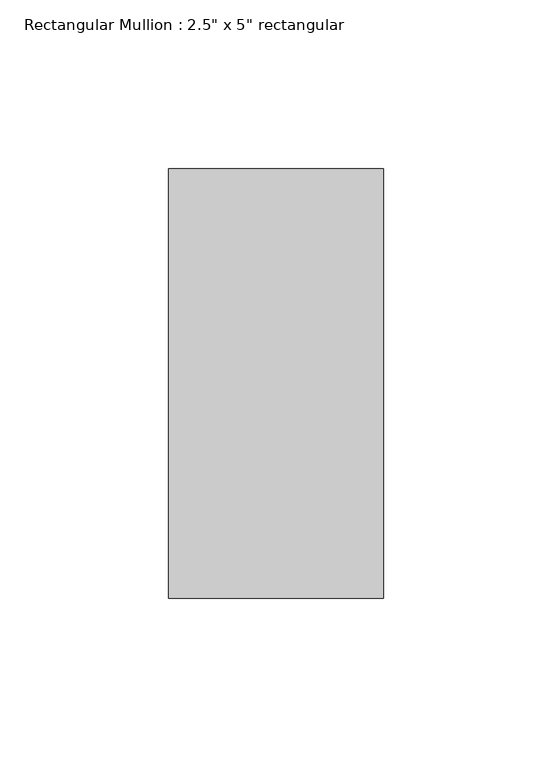
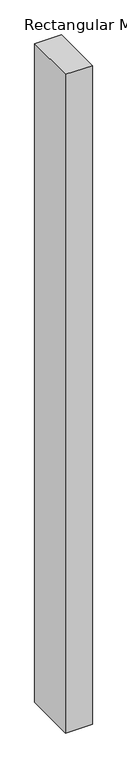
"""IFC4 building model written with IfcOpenShell, lengths in millimetres: member geometry."""

from ifc_helpers import new_model, si_unit, frame, origin, place, context, project, spatial, polyline, outline, extrude, source, transform, mapped, element, save


def member_1e0be150(model_context):
    return source(origin(), model_context, "Body", "SweptSolid", [
        extrude(outline(polyline([(31.75, 63.5), (31.75, -63.5), (-31.75, -63.5), (-31.75, 63.5), (31.75, 63.5)])), frame((0.0, 0.0, -1653.9366569), z_axis=(0.0, 0.0, 1.0), x_axis=(1.0, 0.0, 0.0)), (0.0, 0.0, 1.0), 1653.9366569),
    ])


if __name__ == "__main__":
    model = new_model("IFC4")
    model_context = context("Model", 3, world=origin())
    ifc_project = project(units=[si_unit("LENGTHUNIT", "METRE", prefix="MILLI")], contexts=[model_context])
    site = spatial("IfcSite", under=ifc_project)
    building = spatial("IfcBuilding", under=site)
    placement = place(None, origin())
    member_shape = member_1e0be150(model_context)
    element("IfcMember", 1, ObjectType="Rectangular Mullion : 2.5\" x 5\" rectangular", at=placement, inside=building, context=model_context, shape_type="MappedRepresentation", body=[
        mapped(member_shape, transform((0.0, 0.0, 0.0), x_axis=(1.0, 0.0, 0.0), y_axis=(0.0, 1.0, 0.0), z_axis=(0.0, 0.0, 1.0))),
    ])
    save(model, "model.ifc")

# Revit data of these elements
# Type "Rectangular Mullion : 2.5\" x 5\" rectangular"
#   built-in parameter 1007304 = 0.416667 (stored number, unit not read)
#   built-in parameter 1007301 = 0.104167 (stored number, unit not read)
#   built-in parameter 1007300 = 0.104167 (stored number, unit not read)
# Element 1 (IfcMember, "Rectangular Mullion : 2.5\" x 5\" rectangular")
#   Materials on its faces: "Aluminum"
# Materials
#   "Aluminum": class "Metal", colour RGB 247 247 247, transparency 0, Description = "Aluminum 6061", Cost = 0
